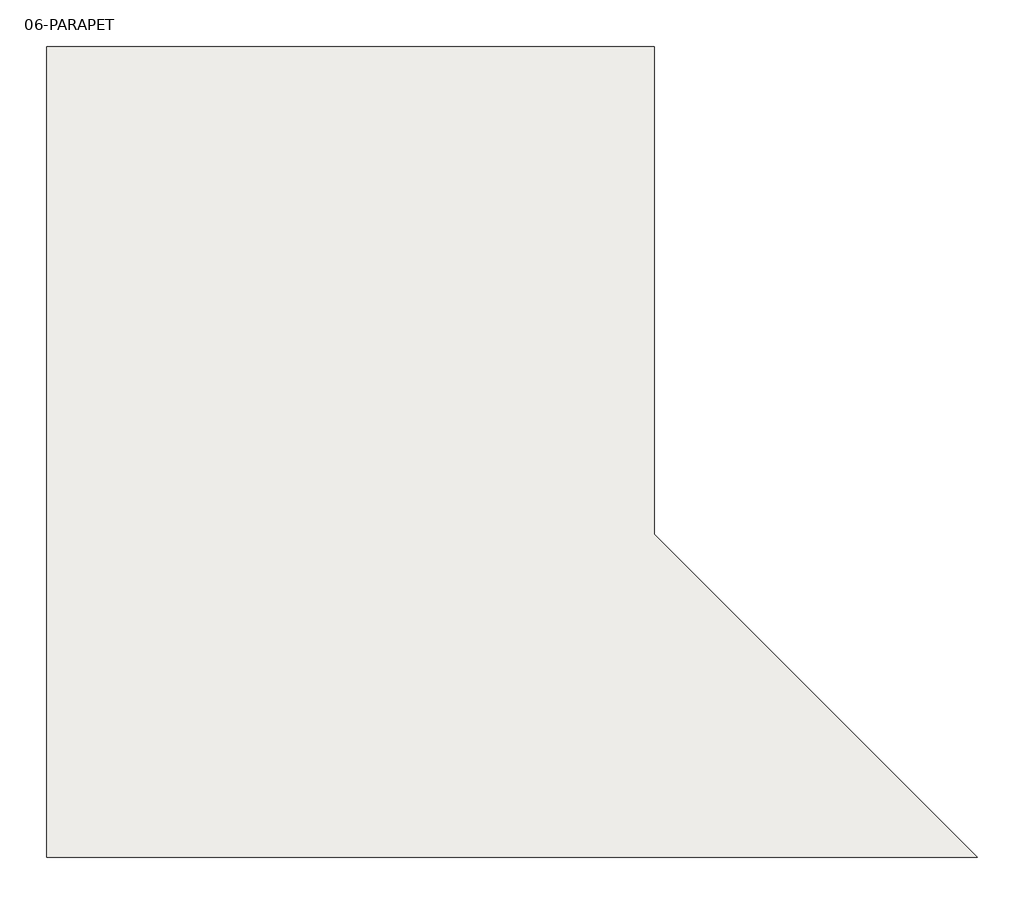
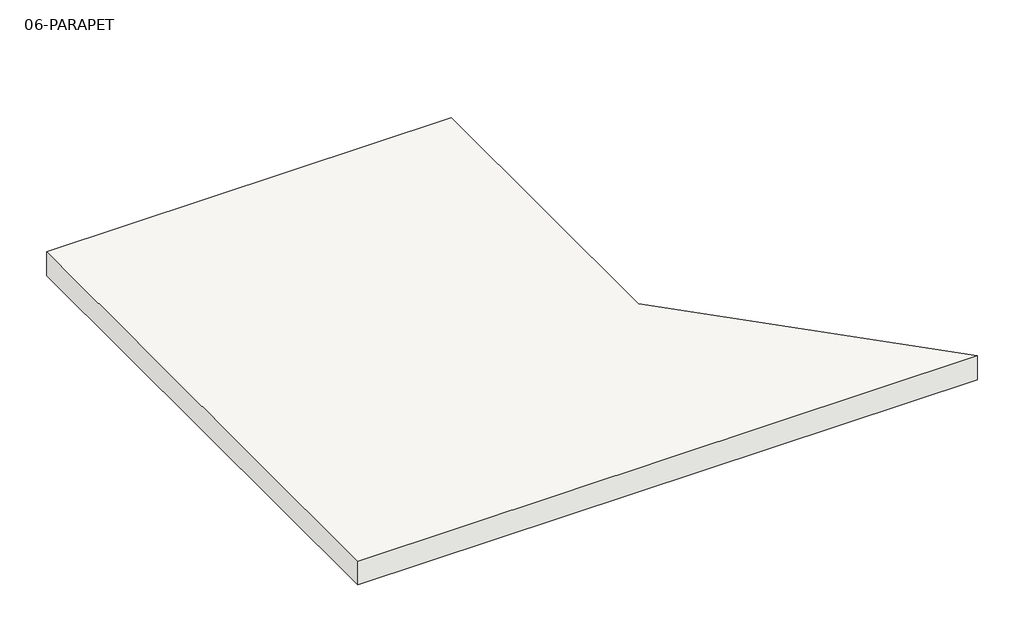
# One storey: 1 slab.
"""IFC4 building model written with IfcOpenShell, lengths in millimetres."""

from ifc_helpers import new_model, si_unit, frame, origin, place, context, project, spatial, polyline, outline, extrude, element, save

model = new_model("IFC4")

# Units and contexts
model_context = context("Model", 3, world=origin())
ifc_project = project(units=[si_unit("LENGTHUNIT", "METRE", prefix="MILLI")], contexts=[model_context])

# Site, building, storey
site = spatial("IfcSite", under=ifc_project)
building = spatial("IfcBuilding", under=site)
storey = spatial("IfcBuildingStorey", under=building, Name="06-PARAPET", Elevation=5550.0)

# Slab
placement = place(None, origin())
element("IfcSlab", 1, ObjectType="02-roof slab", at=placement, inside=storey, context=model_context, shape_type="SweptSolid", body=[
    extrude(outline(polyline([(-3635.4564803, -10622.5265), (-1235.4564803, -10622.5265), (-1235.4564803, -12547.5265), (39.5435197, -13822.5265), (-3635.4564803, -13822.5265), (-3635.4564803, -10622.5265)])), frame((0.0, 0.0, 5700.0), z_axis=(0.0, 0.0, 1.0), x_axis=(1.0, 0.0, 0.0)), (0.0, 0.0, 1.0), 150.0),
])

save(model, "model.ifc")

# Revit data of these elements
# Type "02-roof slab"
#   Description = "Generic Floor (Material By Category), 12\" thick"
#   Assembly Code = "B1010"
#   Type Mark = "G01"
#   Function = 0
#   Layers, outside or top first: 150 mm "concrete floor" (function 1)
# Element 1 (IfcSlab, "02-roof slab")
#   built-in parameter 1001955 = 1.5708 (stored number, unit not read)
#   Height Offset From Level = 300 mm
#   Phase Created = New Construction
#   Materials on its faces: "concrete floor"
# Materials
#   "concrete floor": class "Generic", colour RGB 194 196 182, transparency 0, Cost = 0
